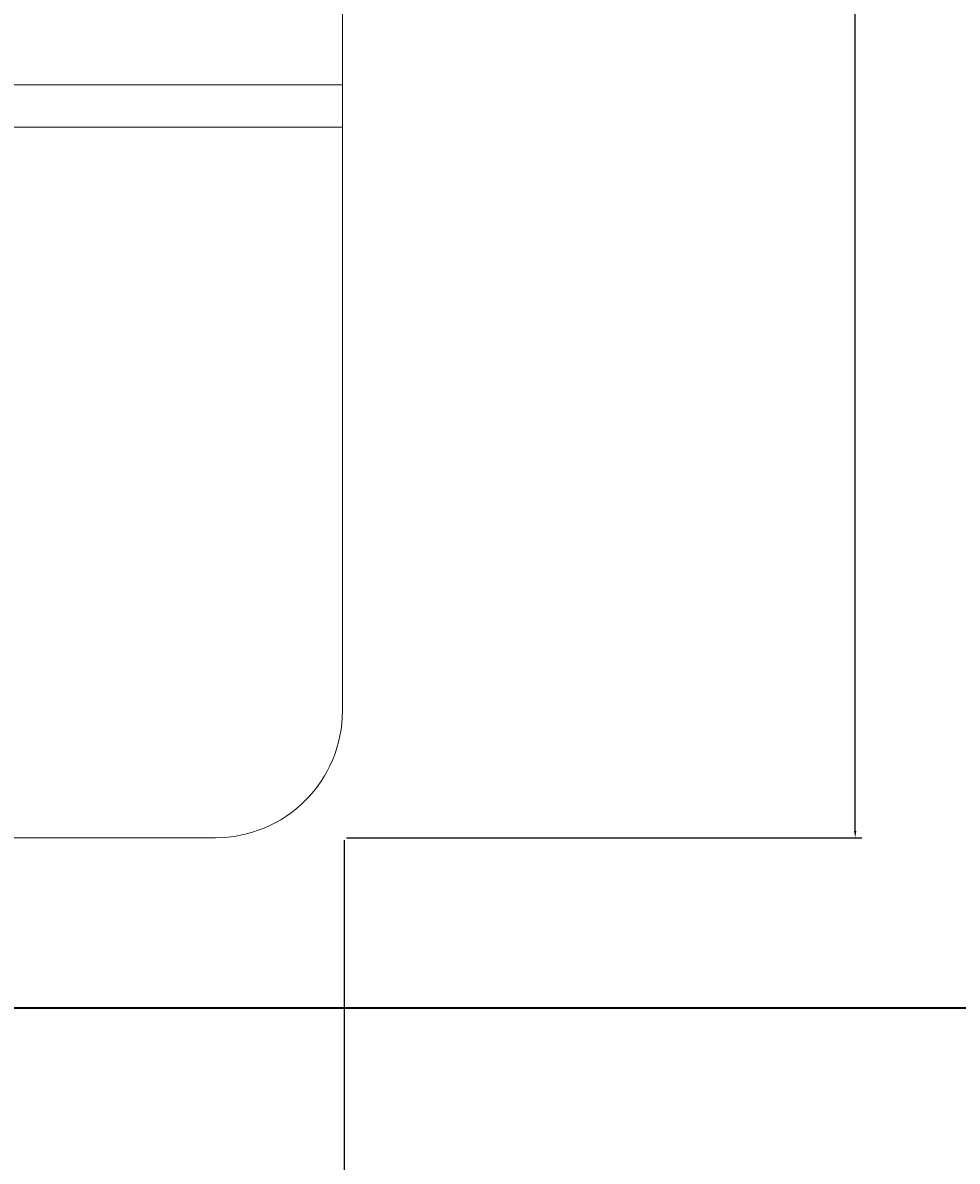
# Model space of a CAD drawing. Units: inches. Extents: x -61 to 1599, y -1316 to 257.
# Tile 8 of 204: x 175 to 200, y -1211 to -1180. Entities that reach past the tile are written whole.
import ezdxf

# ---------------------------------------------------------------- set-up
doc = ezdxf.new("R2010")
doc.units = ezdxf.units.IN
doc.header["$MEASUREMENT"] = 0
for name, color, linetype, lineweight in [('A-ANNO-DIMS', 2, 'Continuous', 18), ('FURNITURE', 83, 'Continuous', 18), ('WALLS', 4, 'Continuous', 35)]:
    doc.layers.add(name, color=color, linetype=linetype, lineweight=lineweight)
doc.styles.get("Standard").update_dxf_attribs({"font": 'arial.ttf'})
doc.dimstyles.get("Standard").update_dxf_attribs({"dimtxt": 0.18, "dimasz": 0.18, "dimexe": 0.18, "dimexo": 0.0625, "dimgap": 0.09, "dimtad": 0, "dimtih": 1, "dimtoh": 1, "dimdec": 0, "dimzin": 0, "dimdsep": 46, "dimlunit": 3, "dimtxsty": 'Standard', "dimcen": 0.09, "dimadec": 0, "dimazin": 0, "dimtfac": 1, "dimtdec": 0, "dimtofl": 0, "dimtmove": 0, "dimatfit": 3, "dimfxl": 1, "dimtolj": 1, "dimtzin": 0, "dimarcsym": 0})

# ---------------------------------------------------------------- blocks, each defined once
blk = doc.blocks.new('BED-DOUBLE')
for p, q in [((1.272, 20.467), (70.263, 20.467)), ((1.272, 19.317), (70.263, 19.317))]:
    blk.add_line(p, q)
blk.add_lwpolyline([(1.272, 88.537), (1.272, 3.449, 0.414214), (4.722, 0), (66.813, 0, 0.414214), (70.263, 3.449), (70.263, 88.537, 0.414214), (66.813, 91.987), (4.722, 91.987, 0.414214)], format="xyb", close=True)
blk = doc.blocks.new('*D634')
at = {"layer": 'A-ANNO-DIMS', "color": 0, "lineweight": -2, "transparency": 16777216}
for p, q in [((183.632, -1109.698), (197.643, -1109.698)), ((197.463, -1109.878), (197.463, -1155.825)), ((197.463, -1202.138), (197.463, -1156.191)), ((183.632, -1202.318), (197.643, -1202.318))]:
    blk.add_line(p, q, dxfattribs=at)
at = {"layer": 'A-ANNO-DIMS', "color": 0, "transparency": 16777216}
for points in [[(197.433, -1109.878), (197.493, -1109.878), (197.463, -1109.698)], [(197.433, -1202.138), (197.493, -1202.138), (197.463, -1202.318)]]:
    blk.add_solid(points, dxfattribs=at)
at = {"layer": 'DEFPOINTS', "color": 0, "transparency": 16777216}
for p in [(183.57, -1109.698), (197.463, -1109.698), (183.57, -1202.318)]:
    blk.add_point(p, dxfattribs=at)
at = {"layer": 'A-ANNO-DIMS', "color": 0, "transparency": 16777216, "insert": (197.463, -1156.008), "char_height": 0.18, "attachment_point": 5}
blk.add_mtext('\\A1;DOUBLE BED 93 TYP.', dxfattribs=at)
blk = doc.blocks.new('*D635')
at = {"layer": 'A-ANNO-DIMS', "color": 0, "lineweight": -2, "transparency": 16777216}
for p, q in [((111.872, -1202.381), (111.872, -1216.391)), ((183.57, -1202.381), (183.57, -1216.391)), ((112.052, -1216.211), (147.193, -1216.211)), ((183.39, -1216.211), (148.248, -1216.211))]:
    blk.add_line(p, q, dxfattribs=at)
at = {"layer": 'A-ANNO-DIMS', "color": 0, "transparency": 16777216}
for points in [[(112.052, -1216.181), (112.052, -1216.241), (111.872, -1216.211)], [(183.39, -1216.181), (183.39, -1216.241), (183.57, -1216.211)]]:
    blk.add_solid(points, dxfattribs=at)
at = {"layer": 'DEFPOINTS', "color": 0, "transparency": 16777216}
for p in [(111.872, -1202.318), (183.57, -1202.318), (183.57, -1216.211)]:
    blk.add_point(p, dxfattribs=at)
at = {"layer": 'A-ANNO-DIMS', "color": 0, "transparency": 16777216, "insert": (147.721, -1216.211), "char_height": 0.18, "attachment_point": 5}
blk.add_mtext('\\A1;72 TYP.', dxfattribs=at)
blk = doc.blocks.new('*D687')
at = {"layer": 'A-ANNO-DIMS', "color": 0, "lineweight": -2, "transparency": 16777216}
for p, q in [((289.418, 181.677), (-61.077, 181.677)), ((-60.897, 181.497), (-60.897, -528.952)), ((-60.897, -1239.765), (-60.897, -529.316)), ((319.64, -1239.945), (-61.077, -1239.945))]:
    blk.add_line(p, q, dxfattribs=at)
at = {"layer": 'A-ANNO-DIMS', "color": 0, "transparency": 16777216}
for points in [[(-60.927, 181.497), (-60.867, 181.497), (-60.897, 181.677)], [(-60.927, -1239.765), (-60.867, -1239.765), (-60.897, -1239.945)]]:
    blk.add_solid(points, dxfattribs=at)
at = {"layer": 'DEFPOINTS', "color": 0, "transparency": 16777216}
for p in [(289.481, 181.677), (-60.897, -1239.945), (319.703, -1239.945)]:
    blk.add_point(p, dxfattribs=at)
at = {"layer": 'A-ANNO-DIMS', "color": 0, "transparency": 16777216, "insert": (-60.897, -529.134), "char_height": 0.18, "attachment_point": 5}
blk.add_mtext('\\A1;1421.6', dxfattribs=at)

msp = doc.modelspace()

# ---------------------------------------------------------------- linework, layer by layer
at = {"layer": 'WALLS'}
msp.add_line((14.7028, -1206.9446), (237.7028, -1206.9446), dxfattribs=at)

# ---------------------------------------------------------------- block references
at = {"layer": 'FURNITURE'}
msp.add_blockref('BED-DOUBLE', (113.2612, -1202.3177), dxfattribs=at)

# ---------------------------------------------------------------- dimensions: what is measured, and where the dimension line sits
at = {"layer": 'A-ANNO-DIMS'}
dim = msp.add_linear_dim(base=(-60.8972, -1239.9446), p1=(289.4807, 181.6771), p2=(319.7028, -1239.9446), angle=90, dimstyle='Standard', override={"dimdec": 1, "dimlfac": 1, "dimrnd": 0, "dimzin": 0, "dimdsep": 46, "dimlunit": 2}, dxfattribs=at)
dim.commit()
dim.dimension.update_dxf_attribs({"geometry": '*D687', "text_midpoint": (-60.8972, -529.1337)})
dim = msp.add_linear_dim(base=(197.4625, -1109.6983), p1=(183.5695, -1202.3182), p2=(183.5695, -1109.6983), angle=90, text='DOUBLE BED <> TYP.', dimstyle='Standard', override={"dimdec": 0, "dimlfac": 1, "dimrnd": 0, "dimzin": 0, "dimdsep": 46, "dimlunit": 2}, dxfattribs=at)
dim.commit()
dim.dimension.update_dxf_attribs({"geometry": '*D634', "text_midpoint": (197.4625, -1156.0082)})
dim = msp.add_linear_dim(base=(183.5695, -1216.2111), p1=(111.8719, -1202.3182), p2=(183.5695, -1202.3182), text='<> TYP.', dimstyle='Standard', override={"dimdec": 0, "dimlfac": 1, "dimrnd": 0, "dimzin": 0, "dimdsep": 46, "dimlunit": 2}, dxfattribs=at)
dim.commit()
dim.dimension.update_dxf_attribs({"geometry": '*D635', "text_midpoint": (147.7207, -1216.2111)})

doc.saveas('drawing.dxf')
